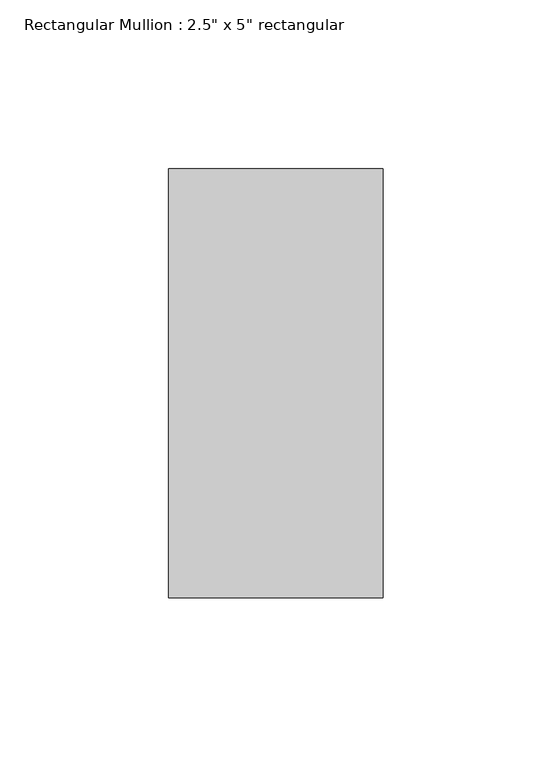
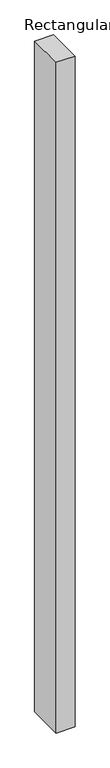
"""IFC4 building model written with IfcOpenShell, lengths in millimetres: member geometry."""

from ifc_helpers import new_model, si_unit, frame, origin, place, context, project, spatial, polyline, outline, extrude, source, transform, mapped, element, save


def member_6afbb202(model_context):
    return source(origin(), model_context, "Body", "SweptSolid", [
        extrude(outline(polyline([(31.75, 63.5), (31.75, -63.5), (-31.75, -63.5), (-31.75, 63.5), (31.75, 63.5)])), frame((0.0, 0.0, -2413.0), z_axis=(0.0, 0.0, 1.0), x_axis=(1.0, 0.0, 0.0)), (0.0, 0.0, 1.0), 2413.0),
    ])


if __name__ == "__main__":
    model = new_model("IFC4")
    model_context = context("Model", 3, world=origin())
    ifc_project = project(units=[si_unit("LENGTHUNIT", "METRE", prefix="MILLI")], contexts=[model_context])
    site = spatial("IfcSite", under=ifc_project)
    building = spatial("IfcBuilding", under=site)
    placement = place(None, origin())
    member_shape = member_6afbb202(model_context)
    element("IfcMember", 1, ObjectType="Rectangular Mullion : 2.5\" x 5\" rectangular", at=placement, inside=building, context=model_context, shape_type="MappedRepresentation", body=[
        mapped(member_shape, transform((0.0, 0.0, 0.0), x_axis=(1.0, 0.0, 0.0), y_axis=(0.0, 1.0, 0.0), z_axis=(0.0, 0.0, 1.0))),
    ])
    save(model, "model.ifc")

# Revit data of these elements
# Type "Rectangular Mullion : 2.5\" x 5\" rectangular"
#   built-in parameter 1007304 = 0.416667 (stored number, unit not read)
#   built-in parameter 1007301 = 0.104167 (stored number, unit not read)
#   built-in parameter 1007300 = 0.104167 (stored number, unit not read)
# Element 1 (IfcMember, "Rectangular Mullion : 2.5\" x 5\" rectangular")
#   Materials on its faces: "Aluminum"
# Materials
#   "Aluminum": class "Metal", colour RGB 247 247 247, transparency 0, Description = "Aluminum 6061", Cost = 0
